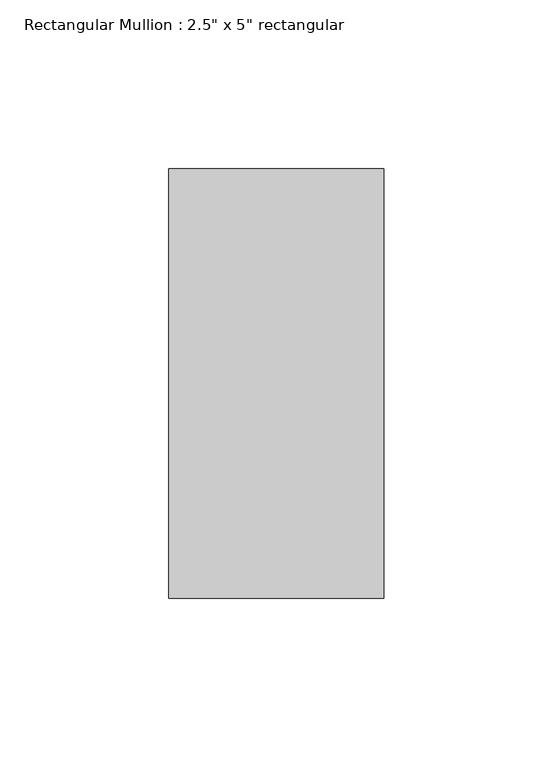
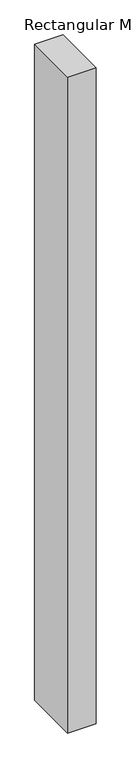
"""IFC4 building model written with IfcOpenShell, lengths in millimetres: member geometry."""

from ifc_helpers import new_model, si_unit, frame, origin, place, context, project, spatial, polyline, outline, extrude, source, transform, mapped, element, save


def member_d87774f7(model_context):
    return source(origin(), model_context, "Body", "SweptSolid", [
        extrude(outline(polyline([(31.75, 63.5), (31.75, -63.5), (-31.75, -63.5), (-31.75, 63.5), (31.75, 63.5)])), frame((0.0, 0.0, -1544.4066766), z_axis=(0.0, 0.0, 1.0), x_axis=(1.0, 0.0, 0.0)), (0.0, 0.0, 1.0), 1544.4066766),
    ])


if __name__ == "__main__":
    model = new_model("IFC4")
    model_context = context("Model", 3, world=origin())
    ifc_project = project(units=[si_unit("LENGTHUNIT", "METRE", prefix="MILLI")], contexts=[model_context])
    site = spatial("IfcSite", under=ifc_project)
    building = spatial("IfcBuilding", under=site)
    placement = place(None, origin())
    member_shape = member_d87774f7(model_context)
    element("IfcMember", 1, ObjectType="Rectangular Mullion : 2.5\" x 5\" rectangular", at=placement, inside=building, context=model_context, shape_type="MappedRepresentation", body=[
        mapped(member_shape, transform((0.0, 0.0, 0.0), x_axis=(1.0, 0.0, 0.0), y_axis=(0.0, 1.0, 0.0), z_axis=(0.0, 0.0, 1.0))),
    ])
    save(model, "model.ifc")

# Revit data of these elements
# Type "Rectangular Mullion : 2.5\" x 5\" rectangular"
#   built-in parameter 1007304 = 0.416667 (stored number, unit not read)
#   built-in parameter 1007301 = 0.104167 (stored number, unit not read)
#   built-in parameter 1007300 = 0.104167 (stored number, unit not read)
# Element 1 (IfcMember, "Rectangular Mullion : 2.5\" x 5\" rectangular")
#   Materials on its faces: "Aluminum"
# Materials
#   "Aluminum": class "Metal", colour RGB 247 247 247, transparency 0, Description = "Aluminum 6061", Cost = 0
